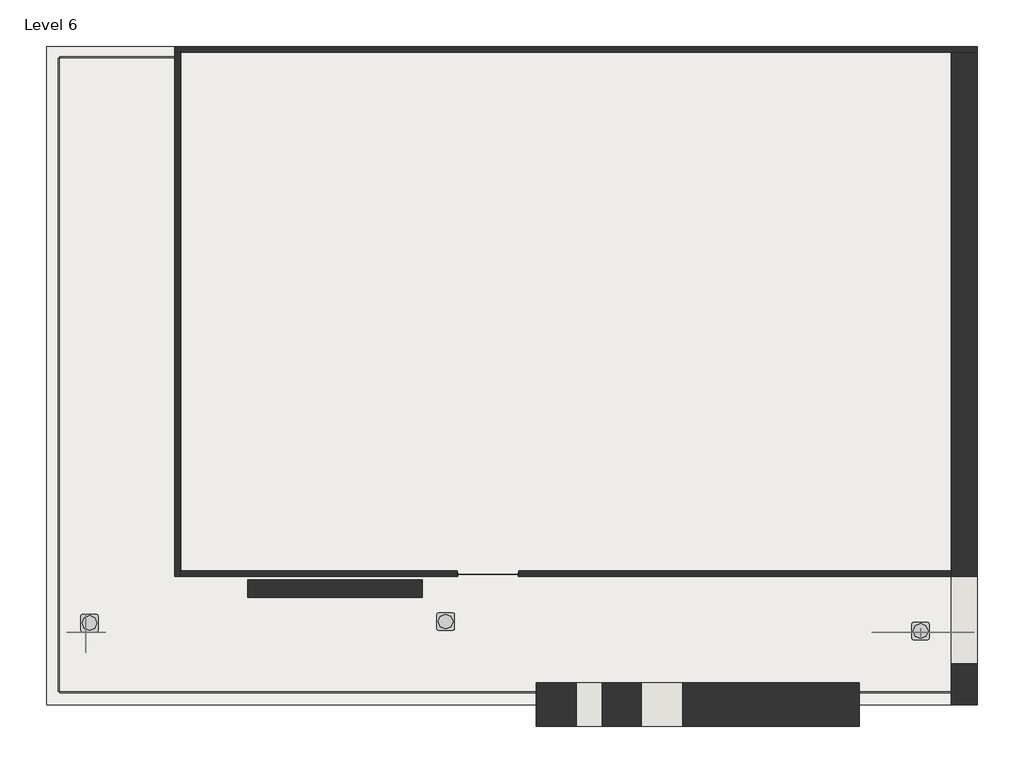
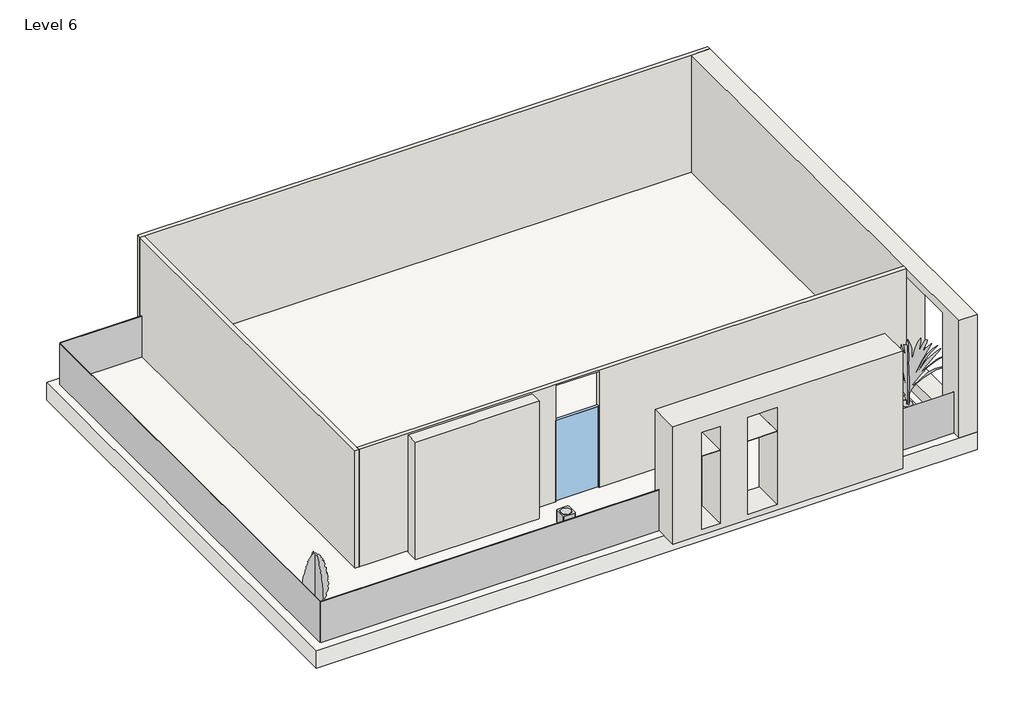
# One storey, incomplete: 6 walls, 4 plates, 3 proxies, 2 geographic elements, 1 slab, 1 window.
"""IFC4 building model written with IfcOpenShell, lengths in millimetres."""

from ifc_helpers import new_model, si_unit, frame, origin, place, context, project, spatial, polyline, outline, extrude, faceted_brep, transform, mapped, element, save
from components import proxy_13b82c07, rpc_tree_conifer_chinese_juniper_7_5155a079, rpc_tree_tropical_0177ab4a, system_panel_glazed_7ce5a3c2, system_panel_glazed_6867f845, system_panel_glazed_ba49168f, system_panel_glazed_c41ca4f4, window_2382273a

model = new_model("IFC4")

# Units and contexts
model_context = context("Model", 3, world=origin())
ifc_project = project(units=[si_unit("LENGTHUNIT", "METRE", prefix="MILLI")], contexts=[model_context])

# Site, building, storey
site = spatial("IfcSite", under=ifc_project)
building = spatial("IfcBuilding", under=site)
storey = spatial("IfcBuildingStorey", under=building, Name="Level 6", Elevation=15240.0)

# Proxies
placement = place(None, origin())
proxy_shape = proxy_13b82c07(model_context)
element("IfcBuildingElementProxy", 1, Name="Air Conditioner-Outside Unit : 33\" x 24\" x 24\"", ObjectType="Air Conditioner-Outside Unit : 33\" x 24\" x 24\"", at=placement, inside=storey, context=model_context, shape_type="MappedRepresentation", body=[
    mapped(proxy_shape, transform((-24603.5874719, -2613.1632813, 14020.8), x_axis=(1.0, 0.0, 0.0), y_axis=(0.0, 1.0, 0.0), z_axis=(0.0, 0.0, 1.0))),
])
element("IfcBuildingElementProxy", 2, Name="Air Conditioner-Outside Unit : 33\" x 24\" x 24\"", ObjectType="Air Conditioner-Outside Unit : 33\" x 24\" x 24\"", at=placement, inside=storey, context=model_context, shape_type="MappedRepresentation", body=[
    mapped(proxy_shape, transform((4377.8125281, -2892.5632813, 14020.8), x_axis=(1.0, 0.0, 0.0), y_axis=(0.0, 1.0, 0.0), z_axis=(0.0, 0.0, 1.0))),
])
element("IfcBuildingElementProxy", 3, Name="Air Conditioner-Outside Unit : 33\" x 24\" x 24\"", ObjectType="Air Conditioner-Outside Unit : 33\" x 24\" x 24\"", at=placement, inside=storey, context=model_context, shape_type="MappedRepresentation", body=[
    mapped(proxy_shape, transform((-12182.9874719, -2562.3632813, 14020.8), x_axis=(1.0, 0.0, 0.0), y_axis=(0.0, 1.0, 0.0), z_axis=(0.0, 0.0, 1.0))),
])

# Geographic elements
rpc_tree_conifer_chinese_juniper_7_shape = rpc_tree_conifer_chinese_juniper_7_5155a079(model_context)
element("IfcGeographicElement", 4, ObjectType="RPC Tree - Conifer : Chinese Juniper - 7'", at=placement, inside=storey, context=model_context, shape_type="MappedRepresentation", body=[
    mapped(rpc_tree_conifer_chinese_juniper_7_shape, transform((-24730.784143, -2943.3632813, 14020.8), x_axis=(1.0, 0.0, 0.0), y_axis=(0.0, 1.0, 0.0), z_axis=(0.0, 0.0, 1.0))),
])
rpc_tree_tropical_shape = rpc_tree_tropical_0177ab4a(model_context)
element("IfcGeographicElement", 5, ObjectType="RPC Tree - Tropical", at=placement, inside=storey, context=model_context, shape_type="MappedRepresentation", body=[
    mapped(rpc_tree_tropical_shape, transform((4377.8125281, -2943.3632813, 14020.8), x_axis=(1.0, 0.0, 0.0), y_axis=(0.0, 1.0, 0.0), z_axis=(0.0, 0.0, 1.0))),
])

# Plates
system_panel_glazed_shape = system_panel_glazed_7ce5a3c2(model_context)
element("IfcPlate", 6, ObjectType="System Panel : Glazed", at=placement, inside=storey, context=model_context, shape_type="MappedRepresentation", body=[
    mapped(system_panel_glazed_shape, transform((3844.4125281, -5000.7632813, 14020.8), x_axis=(-1.0, 0.0, 0.0), y_axis=(0.0, -1.0, 0.0), z_axis=(0.0, 0.0, 1.0))),
])
system_panel_glazed_2_shape = system_panel_glazed_6867f845(model_context)
element("IfcPlate", 7, ObjectType="System Panel : Glazed", at=placement, inside=storey, context=model_context, shape_type="MappedRepresentation", body=[
    mapped(system_panel_glazed_2_shape, transform((-17339.1874719, -5000.7632813, 14020.8), x_axis=(-1.0, 0.0, 0.0), y_axis=(0.0, -1.0, 0.0), z_axis=(0.0, 0.0, 1.0))),
])
system_panel_glazed_3_shape = system_panel_glazed_ba49168f(model_context)
element("IfcPlate", 8, ObjectType="System Panel : Glazed", at=placement, inside=storey, context=model_context, shape_type="MappedRepresentation", body=[
    mapped(system_panel_glazed_3_shape, transform((-25644.9874719, 6048.2367187, 14020.8), x_axis=(0.0, 1.0, 0.0), y_axis=(-1.0, 0.0, 0.0), z_axis=(0.0, 0.0, 1.0))),
])
system_panel_glazed_4_shape = system_panel_glazed_c41ca4f4(model_context)
element("IfcPlate", 9, ObjectType="System Panel : Glazed", at=placement, inside=storey, context=model_context, shape_type="MappedRepresentation", body=[
    mapped(system_panel_glazed_4_shape, transform((-23638.3874719, 17097.2367187, 14020.8), x_axis=(1.0, 0.0, 0.0), y_axis=(0.0, 1.0, 0.0), z_axis=(0.0, 0.0, 1.0))),
])

# Slab
element("IfcSlab", 10, ObjectType="Generic - 3'", at=placement, inside=storey, context=model_context, shape_type="SweptSolid", body=[
    extrude(outline(polyline([(-26102.1874719, -5457.9632813), (-26102.1874719, 17503.6367187), (6359.0125281, 17503.6367187), (6359.0125281, -5457.9632813), (-26102.1874719, -5457.9632813)])), frame((0.0, 0.0, 13106.4), z_axis=(0.0, 0.0, 1.0), x_axis=(1.0, 0.0, 0.0)), (0.0, 0.0, 1.0), 914.4),
])

# Walls
element("IfcWall", 11, ObjectType="Generic - 3'", at=placement, inside=storey, context=model_context, shape_type="Brep", body=[
    faceted_brep([(5444.6125281, 17300.4367187, 14020.8), (5444.6125281, -784.3632813, 14020.8), (5444.6125281, -987.5632813, 14020.8), (5444.6125281, -5457.9632813, 14020.8), (5444.6125281, -5457.9632813, 20116.8), (5444.6125281, -987.5632813, 20116.8), (5444.6125281, -784.3632813, 20116.8), (5444.6125281, 17300.4367187, 20116.8), (5444.6125281, -4035.5632813, 19669.287938), (5444.6125281, -4035.5632813, 14640.087938), (5444.6125281, -987.5632813, 14640.087938), (5444.6125281, -987.5632813, 19669.287938), (6359.0125281, 17300.4367187, 14020.8), (6359.0125281, 17300.4367187, 20116.8), (6359.0125281, -5457.9632813, 20116.8), (6359.0125281, -5457.9632813, 14020.8), (6359.0125281, -4035.5632813, 19669.287938), (6359.0125281, -987.5632813, 19669.287938), (6359.0125281, -987.5632813, 14640.087938), (6359.0125281, -4035.5632813, 14640.087938)], [[[0, 1, 2, 3, 4, 5, 6, 7], [8, 9, 10, 11]], [[12, 13, 14, 15], [16, 17, 18, 19]], [[0, 7, 13, 12]], [[3, 2, 1, 0, 12, 15]], [[4, 3, 15, 14]], [[7, 6, 5, 4, 14, 13]], [[9, 8, 16, 19]], [[10, 9, 19, 18]], [[8, 11, 17, 16]], [[11, 10, 18, 17]]]),
])
element("IfcWall", 12, ObjectType="Generic - 3' gray", at=placement, inside=storey, context=model_context, shape_type="SweptSolid", body=[
    extrude(outline(polyline([(14020.8, 2244.2125281), (20116.8, 2244.2125281), (20116.8, -9033.3874719), (14020.8, -9033.3874719), (14020.8, 2244.2125281)]), holes=[polyline([(19336.1308744, -6716.0306948), (18116.9308744, -6716.0306948), (18116.9308744, -7630.4306948), (19336.1308744, -7630.4306948), (19336.1308744, -6716.0306948)]), polyline([(14306.9308744, -7630.4306948), (18091.5308744, -7630.4306948), (18091.5308744, -6716.0306948), (14306.9308744, -6716.0306948), (14306.9308744, -7630.4306948)]), polyline([(19336.1308744, -3924.8577662), (18116.9308744, -3924.8577662), (18116.9308744, -5371.4183212), (19336.1308744, -5371.4183212), (19336.1308744, -3924.8577662)]), polyline([(14306.9308744, -5371.4183212), (18091.5308744, -5371.4183212), (18091.5308744, -3924.8577662), (14306.9308744, -3924.8577662), (14306.9308744, -5371.4183212)])]), frame((0.0, -6219.9632813, 0.0), z_axis=(0.0, 1.0, 0.0), x_axis=(0.0, 0.0, 1.0)), (0.0, 0.0, 1.0), 1524.0),
])
element("IfcWall", 13, ObjectType="Generic - 8\"", at=placement, inside=storey, context=model_context, shape_type="Brep", body=[
    faceted_brep([(-21631.7874719, 17300.4367187, 14020.8), (-21428.5874719, 17300.4367187, 14020.8), (5444.6125281, 17300.4367187, 14020.8), (6359.0125281, 17300.4367187, 14020.8), (6359.0125281, 17300.4367187, 20116.8), (5444.6125281, 17300.4367187, 20116.8), (-21428.5874719, 17300.4367187, 20116.8), (-21631.7874719, 17300.4367187, 20116.8), (-21631.7874719, 17503.6367187, 14020.8), (-21631.7874719, 17503.6367187, 20116.8), (6359.0125281, 17503.6367187, 20116.8), (6359.0125281, 17503.6367187, 14020.8)], [[[0, 1, 2, 3, 4, 5, 6, 7]], [[8, 9, 10, 11]], [[3, 2, 1, 0, 8, 11]], [[7, 6, 5, 4, 10, 9]], [[0, 7, 9, 8]], [[4, 3, 11, 10]]]),
])
element("IfcWall", 14, ObjectType="Generic - 8\"", at=placement, inside=storey, context=model_context, shape_type="Brep", body=[
    faceted_brep([(-21428.5874719, -987.5632813, 14020.8), (-21428.5874719, -784.3632813, 14020.8), (-21428.5874719, 17300.4367187, 14020.8), (-21428.5874719, 17300.4367187, 20116.8), (-21428.5874719, -784.3632813, 20116.8), (-21428.5874719, -987.5632813, 20116.8), (-21631.7874719, -987.5632813, 14020.8), (-21631.7874719, -987.5632813, 20116.8), (-21631.7874719, 17300.4367187, 20116.8), (-21631.7874719, 17300.4367187, 14020.8)], [[[0, 1, 2, 3, 4, 5]], [[6, 7, 8, 9]], [[2, 1, 0, 6, 9]], [[5, 4, 3, 8, 7]], [[0, 5, 7, 6]], [[3, 2, 9, 8]]]),
])
element("IfcWall", 15, ObjectType="Generic - 8\"", at=placement, inside=storey, context=model_context, shape_type="Brep", body=[
    faceted_brep([(-21428.5874719, -784.3632813, 20116.8), (5444.6125281, -784.3632813, 20116.8), (5444.6125281, -784.3632813, 14020.8), (-9642.9874719, -784.3632813, 14020.8), (-9642.9874719, -784.3632813, 20055.4483945), (-11776.5874719, -784.3632813, 20055.4483945), (-11776.5874719, -784.3632813, 14020.8), (-21428.5874719, -784.3632813, 14020.8), (5444.6125281, -987.5632813, 20116.8), (-21428.5874719, -987.5632813, 20116.8), (-21428.5874719, -987.5632813, 14020.8), (-11776.5874719, -987.5632813, 14020.8), (-11776.5874719, -987.5632813, 20055.4483945), (-9642.9874719, -987.5632813, 20055.4483945), (-9642.9874719, -987.5632813, 14020.8), (5444.6125281, -987.5632813, 14020.8), (5444.6125281, -987.5632813, 14640.087938), (5444.6125281, -987.5632813, 19669.287938)], [[[0, 1, 2, 3, 4, 5, 6, 7]], [[8, 9, 10, 11, 12, 13, 14, 15, 16, 17]], [[10, 7, 6, 11]], [[3, 2, 15, 14]], [[1, 0, 9, 8]], [[0, 7, 10, 9]], [[11, 6, 5, 12]], [[3, 14, 13, 4]], [[12, 5, 4, 13]], [[15, 2, 1, 8, 17, 16]]]),
])
element("IfcWall", 16, ObjectType="Generic -2", at=placement, inside=storey, context=model_context, shape_type="SweptSolid", body=[
    extrude(outline(polyline([(-12995.7874719, -1724.1632813), (-19091.7874719, -1724.1632813), (-19091.7874719, -1114.5632813), (-12995.7874719, -1114.5632813), (-12995.7874719, -1724.1632813)])), frame((0.0, 0.0, 14020.8), z_axis=(0.0, 0.0, 1.0), x_axis=(1.0, 0.0, 0.0)), (0.0, 0.0, 1.0), 6106.1211964),
])

# Window
window_shape = window_2382273a(model_context)
element("IfcWindow", 17, ObjectType="Instance - Fixed : 24\" x 48\"", at=placement, inside=storey, context=model_context, shape_type="MappedRepresentation", body=[
    mapped(window_shape, transform((-10747.8874719, -885.9632813, 13078.255451), x_axis=(-1.0, 0.0, 0.0), y_axis=(0.0, -1.0, 0.0), z_axis=(0.0, 0.0, 1.0))),
])

save(model, "model.ifc")

# Revit data of these elements
# Type "Air Conditioner-Outside Unit : 33\" x 24\" x 24\""
#   Assembly Code = "D3030"
#   Depth = 2' - 0"
#   Height = 2' - 0"
#   Width = 2' - 0"
#   Air Conditioner Material = Steel, Paint Finish, Dark Gray, Matte
#   Default Elevation = 0
# Type "RPC Tree - Conifer : Chinese Juniper - 7'"
#   built-in parameter 1005198 = "{2, 15},{39, RPC-16-FUM3-UUQ0-UBF0-N000-ST1L-LVER-AU},{1, 0},{1, 0},{2, 13},{1, 8},{5, Color},{1, 0},{1, 0},{3, 0.8},{3, 0.8},{3, 0.8},{1, 8},{7, BBoxMin},{1, 0},{1, 0},{1, 0},{1, 0},{1, 0},{1, 8},{7, BBoxMax},{1, 0},{1, 0},{1, 0},{1, 0},{1, 0},{2, 11},{9, RPCTypeId},{1, 0},{1, 0},{39, RPC-16-FUM3-UUQ0-UBF0-N000-ST1L-LVER-AU},{1, 6},{14, RPCPlantHeight},{1, 0},{1, 0},{1, 7},{2, 11},{7, keyword},{1, 0},{1, 0},{34, :RPCs:Trees [General]:Geometry:RPC},{2, 11},{8, category},{1, 0},{1, 0},{15, Trees [General]},{2, 11},{12, LocalizedUID},{1, 0},{1, 0},{15, Chinese Juniper},{2, 14},{6, Height},{1, 0},{1, 0},{1, 7},{1, 2},{16, Cast Reflections},{1, 0},{1, 0},{1, 0},{1, 2},{12, Cast Shadows},{1, 0},{1, 0},{1, 1},{1, 2},{9, Lock View},{1, 0},{1, 0},{1, 0},{1, 4},{5, ViewC},{1, 0},{1, 0},{1, 0},{21, assetlibrary_base.fbx},{1, 5},"
#   built-in parameter 1005195 = "RPC-16-FUM3-UUQ0-UBF0-N000-ST1L-LVER-AU"
#   Type Comments = "Chinese Juniper"
#   Assembly Code = "G2050500"
#   Height = 10' - 0"
#   Description = (empty or 0)
#   Default Elevation = 0
# Type "RPC Tree - Tropical"
#   built-in parameter 1005198 = "{2, 15},{39, RPC-16-G2M6-EAFX-C5H6-W000-ST1L-LVER-AU},{1, 0},{1, 0},{2, 13},{1, 8},{5, Color},{1, 0},{1, 0},{3, 0.8},{3, 0.8},{3, 0.8},{1, 8},{7, BBoxMin},{1, 0},{1, 0},{1, 0},{1, 0},{1, 0},{1, 8},{7, BBoxMax},{1, 0},{1, 0},{1, 0},{1, 0},{1, 0},{2, 11},{9, RPCTypeId},{1, 0},{1, 0},{39, RPC-16-G2M6-EAFX-C5H6-W000-ST1L-LVER-AU},{1, 6},{14, RPCPlantHeight},{1, 0},{1, 0},{2, 13},{2, 11},{7, keyword},{1, 0},{1, 0},{35, :RPCs:Trees [Tropical]:Geometry:RPC},{2, 11},{8, category},{1, 0},{1, 0},{16, Trees [Tropical]},{2, 11},{12, LocalizedUID},{1, 0},{1, 0},{15, Traveler's Palm},{2, 14},{6, Height},{1, 0},{1, 0},{2, 13},{1, 2},{16, Cast Reflections},{1, 0},{1, 0},{1, 0},{1, 2},{12, Cast Shadows},{1, 0},{1, 0},{1, 1},{1, 2},{9, Lock View},{1, 0},{1, 0},{1, 0},{1, 4},{5, ViewC},{1, 0},{1, 0},{1, 0},{21, assetlibrary_base.fbx},{1, 5},"
#   built-in parameter 1005195 = "RPC-16-G2M6-EAFX-C5H6-W000-ST1L-LVER-AU"
#   Assembly Code = "G2050500"
#   Height = 13' - 0"
#   Plan Symbol = element 321958
#   Default Elevation = 0
# Type "System Panel : Glazed"
#   Construction Type Id = "GSP4R"
#   Analytic Construction = "1/8 in Pilkington single glazing"
#   Visual Light Transmittance = 0.9
#   Solar Heat Gain Coefficient = 0.86
#   Heat Transfer Coefficient (U) = 1.18115 BTU/(h·ft²·°F)
# Type "Generic - 3'"
#   Assembly Code = "B1010"
#   Function = 0
#   Layers, outside or top first: 3' - 0" "Parking Stripe" (function 1)
# Type "Generic - 3'"
#   Assembly Code = "B2010"
#   Layers, outside or top first: 3' - 0" "Parking Stripe" (function 1)
# Type "Generic - 3' gray"
#   Assembly Code = "B2010"
#   Layers, outside or top first: 5' - 0" "Concrete, Lightweight" (function 1)
# Type "Generic - 8\""
#   Assembly Code = "B2010"
#   Layers, outside or top first: 0' - 8" no material (function 1)
# Type "Generic -2"
#   Assembly Code = "B2010"
#   Layers, outside or top first: 2' - 0" "Plywood, Sheathing" (function 1)
# Type "Instance - Fixed : 24\" x 48\""
#   Type Mark = "10"
#   Construction Type Id = "GSP4R"
#   Assembly Code = "B2020100"
#   Analytic Construction = "1/8 in Pilkington single glazing"
#   Visual Light Transmittance = 0.9
#   Thermal Resistance (R) = 0.8466 (h·ft²·°F)/BTU
#   Solar Heat Gain Coefficient = 0.86
#   Heat Transfer Coefficient (U) = 1.1812 BTU/(h·ft²·°F)
#   Height [instance default] = 4' - 0"
#   Default Sill Height = 3' - 0"
#   Width [instance default] = 2' - 0"
#   Window Inset = 0' - 2"
#   Define Thermal Properties by = 1
#   Glass Pane Material = Glass
#   Sash Material = Iron, Ductile
#   Wall Closure = (empty or 0)
# Element 1 (IfcBuildingElementProxy, "Air Conditioner-Outside Unit : 33\" x 24\" x 24\"")
#   Mark = "7"
#   Phase Created = New Construction
#   Materials on its faces: "Steel, Paint Finish, Dark Gray, Matte"
# Element 2 (IfcBuildingElementProxy, "Air Conditioner-Outside Unit : 33\" x 24\" x 24\"")
#   Mark = "8"
#   Phase Created = New Construction
#   Materials on its faces: "Steel, Paint Finish, Dark Gray, Matte"
# Element 3 (IfcBuildingElementProxy, "Air Conditioner-Outside Unit : 33\" x 24\" x 24\"")
#   Mark = "9"
#   Phase Created = New Construction
#   Materials on its faces: "Steel, Paint Finish, Dark Gray, Matte"
# Element 4 (IfcGeographicElement, "RPC Tree - Conifer : Chinese Juniper - 7'")
#   Phase Created = New Construction
# Element 5 (IfcGeographicElement, "RPC Tree - Tropical")
#   Phase Created = New Construction
# Elements 6, 7, 8, 9 (IfcPlate, "System Panel : Glazed")
#   Phase Created = New Construction
#   Materials on its faces: "Glass"
# Element 10 (IfcSlab, "Generic - 3'")
#   built-in parameter 1001955 = 3.14159 (stored number, unit not read)
#   Height Offset From Level = -4' - 0"
#   Phase Created = New Construction
#   Materials on its faces: "Parking Stripe"
# Element 11 (IfcWall, "Generic - 3'")
#   built-in parameter 1001111 = -4' - 0"
#   Top Offset = 0' - 0"
#   Base Offset = -4' - 0"
#   Unconnected Height = 20' - 0"
#   wall height = 20' - 0"
#   Phase Created = New Construction
#   Base Constraint = Level 6
#   Materials on its faces: "Parking Stripe", "Default Wall"
# Element 12 (IfcWall, "Generic - 3' gray")
#   built-in parameter 1001111 = -4' - 0"
#   Top Offset = 0' - 0"
#   Base Offset = -4' - 0"
#   Unconnected Height = 20' - 0"
#   wall height = 20' - 0"
#   Phase Created = New Construction
#   Base Constraint = Level 6
#   Materials on its faces: "Concrete, Lightweight"
# Element 13 (IfcWall, "Generic - 8\"")
#   built-in parameter 1001111 = -4' - 0"
#   Top Offset = 0' - 0"
#   Base Offset = -4' - 0"
#   Unconnected Height = 20' - 0"
#   wall height = 20' - 0"
#   Phase Created = New Construction
#   Base Constraint = Level 6
#   Materials on its faces: "Default Wall", "Parking Stripe"
# Elements 14, 15 (IfcWall, "Generic - 8\"")
#   built-in parameter 1001111 = -4' - 0"
#   Top Offset = 0' - 0"
#   Base Offset = -4' - 0"
#   Unconnected Height = 20' - 0"
#   wall height = 20' - 0"
#   Phase Created = New Construction
#   Base Constraint = Level 6
#   Materials on its faces: "Default Wall"
# Element 16 (IfcWall, "Generic -2")
#   built-in parameter 1001111 = -4' - 0"
#   Top Offset = 0' - 0"
#   Base Offset = -4' - 0"
#   Unconnected Height = 20' - 0.39847"
#   wall height = 20' - 0.39847"
#   Phase Created = New Construction
#   Base Constraint = Level 6
#   Materials on its faces: "Plywood, Sheathing"
# Element 17 (IfcWindow, "Instance - Fixed : 24\" x 48\"")
#   Mark = "5"
#   Width = 7' - 0"
#   Height = 14' - 0"
#   Phase Created = New Construction
#   Materials on its faces: "Iron, Ductile", "Glass"
# Materials
#   "Steel, Paint Finish, Dark Gray, Matte": class "Metal", colour RGB 98 98 98, transparency 0, Description = "Steel, paint finish, dark gray, matte", Cost = 0
#   "Parking Stripe": class "Paint", colour RGB 250 250 91, transparency 0, Cost = 0
#   "Concrete, Lightweight": class "Concrete", colour RGB 142 141 140, transparency 0, Description = "Lightweight concrete", Cost = 0
#   "Plywood, Sheathing": class "Wood", colour RGB 212 179 113, transparency 0, Description = "Plywood, sheathing grade", Cost = 0
#   "Glass": class "Glass", colour RGB 0 128 192, transparency 0.75, Description = "Soda Lime Glass", Cost = 0
#   "Iron, Ductile": class "Metal", colour RGB 0 0 0, transparency 0, Description = "Ductile cast iron", Cost = 0
#   "Default Wall": colour RGB 128 128 128, transparency 0
